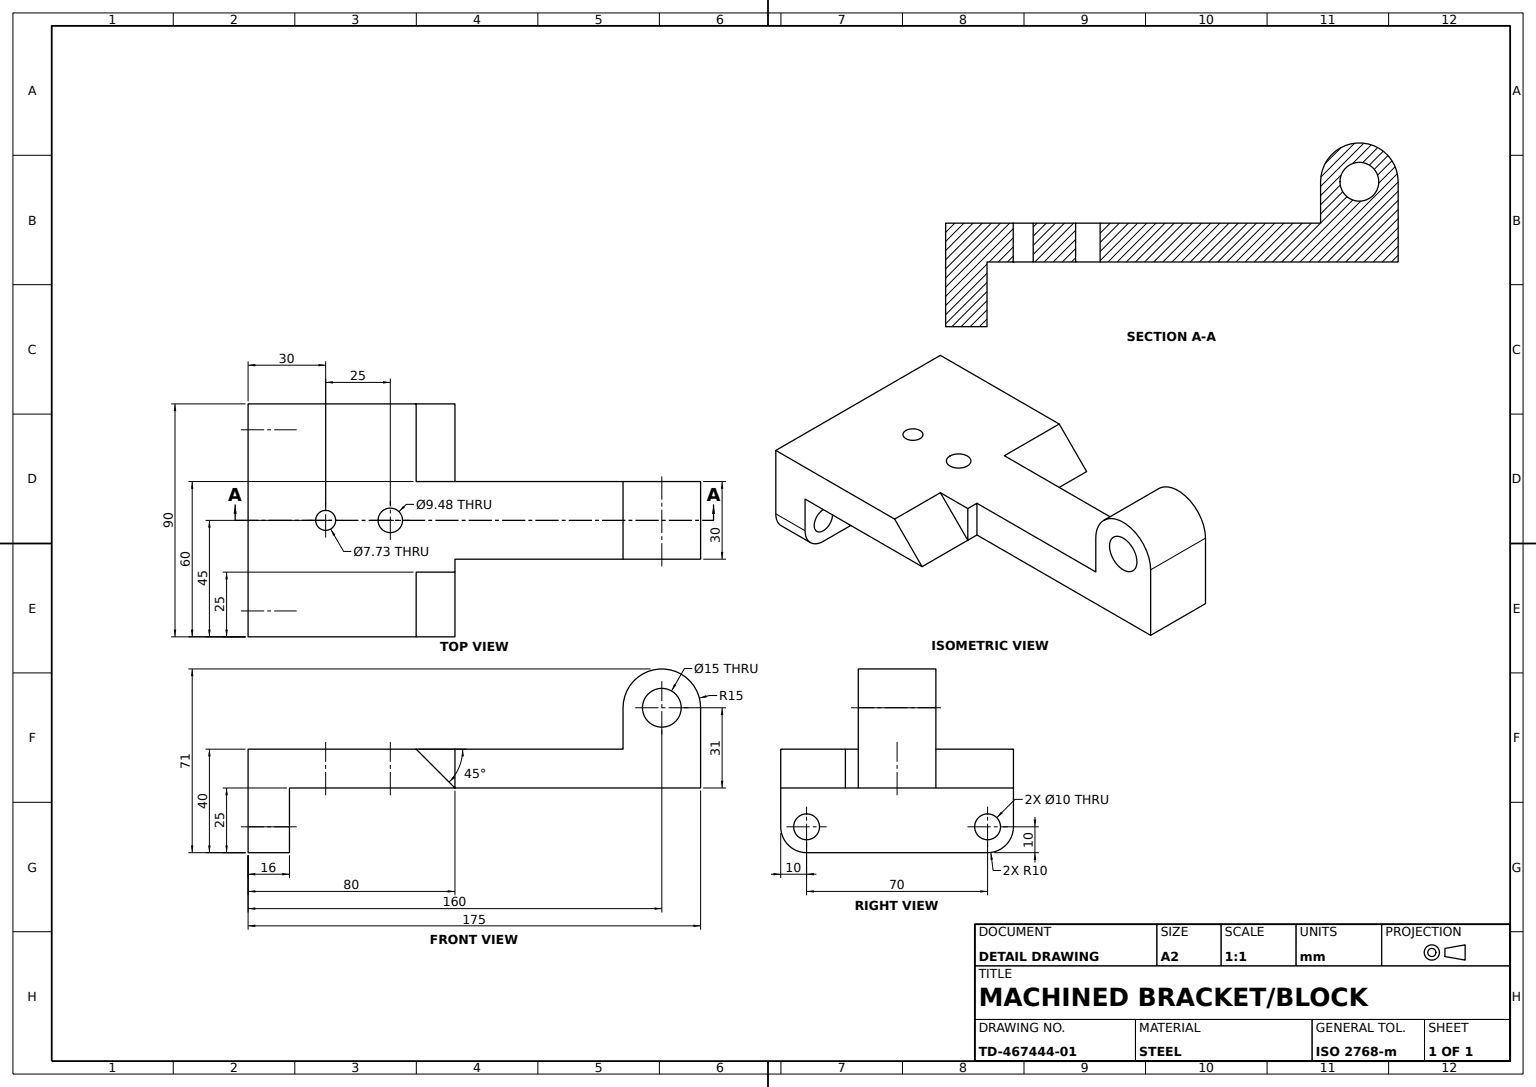
from build123d import *

# Parameters (mm, degrees)
BASE_BLOCK_DEPTH        = 45
STEP_BOSS_PROFILE_W     = 15
STEP_BOSS_PROFILE_H     = 35
STEP_BOSS_DEPTH         = 15
ARM_PROFILE_W           = 30
ARM_PROFILE_H           = 15
EXTENSION_ARM_DEPTH     = 95
HINGE_LUG_PROFILE_R     = 7.5
HINGE_LUG_DEPTH         = 30
EDGE_FILLET_R10_R       = 10
PIN_HOLES_PROFILE_R     = 5
PIN_HOLES_THROUGH_DEPTH = 60
TOP_HOLES_PROFILE_R     = 3.862710878
TOP_HOLES_PROFILE_R_2   = 4.740282405
TOP_HOLES_THROUGH_DEPTH = 60


with BuildPart() as part:
    # Base Block Profile → Base Block (new, symmetric)
    with BuildSketch(Plane.XY):
        Polygon((0, 0), (0, -40), (16, -40), (16, -15), (80, -15), (65, 0), align=None)
    extrude(amount=BASE_BLOCK_DEPTH, both=True)

    # Step Boss Profile → Step Boss (add)
    with BuildSketch(Plane(origin=(0, 0, 0), x_dir=(1, 0, 0), z_dir=(0, 1, 0))):
        with Locations((72.5, -2.5)):
            Rectangle(STEP_BOSS_PROFILE_W, STEP_BOSS_PROFILE_H)
    extrude(amount=-STEP_BOSS_DEPTH)

    # Arm Profile → Extension Arm (add)
    with BuildSketch(Plane(origin=(80, 0, 0), x_dir=(0, 0, -1), z_dir=(1, 0, 0))):
        with Locations((0, -7.5)):
            Rectangle(ARM_PROFILE_W, ARM_PROFILE_H)
    extrude(amount=EXTENSION_ARM_DEPTH)

    # Hinge Lug Profile → Hinge Lug (add)
    with BuildSketch(Plane.XY.offset(15)):
        with BuildLine():
            Line((145, 16), (145, -10.792045984))
            Line((145, -10.792045984), (175, -10.792045984))
            Line((175, -10.792045984), (175, 16))
            ThreePointArc((175, 16), (160, 31), (145, 16))
        make_face()
        with Locations((160, 16)):
            Circle(HINGE_LUG_PROFILE_R, mode=Mode.SUBTRACT)
    extrude(amount=-HINGE_LUG_DEPTH)

    # Edge Fillet R10
    edge_fillet_r10_edges = [part.edges().sort_by_distance(p)[0] for p in [
        (8, -40, 45),
        (8, -40, -45),
    ]]
    fillet(edge_fillet_r10_edges, radius=EDGE_FILLET_R10_R)

    # Pin Holes Profile → Pin Holes Through (cut, symmetric)
    with BuildSketch(Plane.ZY):
        with Locations(Location((-35, -30, 0), (0, 0, 270))):
            Circle(PIN_HOLES_PROFILE_R)
        with Locations(Location((35, -30, 0), (0, 0, 270))):
            Circle(PIN_HOLES_PROFILE_R)
    extrude(amount=PIN_HOLES_THROUGH_DEPTH, both=True, mode=Mode.SUBTRACT)

    # Top Holes Profile → Top Holes Through (cut, symmetric)
    with BuildSketch(Plane(origin=(0, 0, 0), x_dir=(1, 0, 0), z_dir=(0, 1, 0))):
        with Locations(Location((30, 0, 0), (0, 0, 180))):
            Circle(TOP_HOLES_PROFILE_R)
        with Locations(Location((55, 0, 0), (0, 0, 180))):
            Circle(TOP_HOLES_PROFILE_R_2)
    extrude(amount=TOP_HOLES_THROUGH_DEPTH, both=True, mode=Mode.SUBTRACT)


solid = part.part
